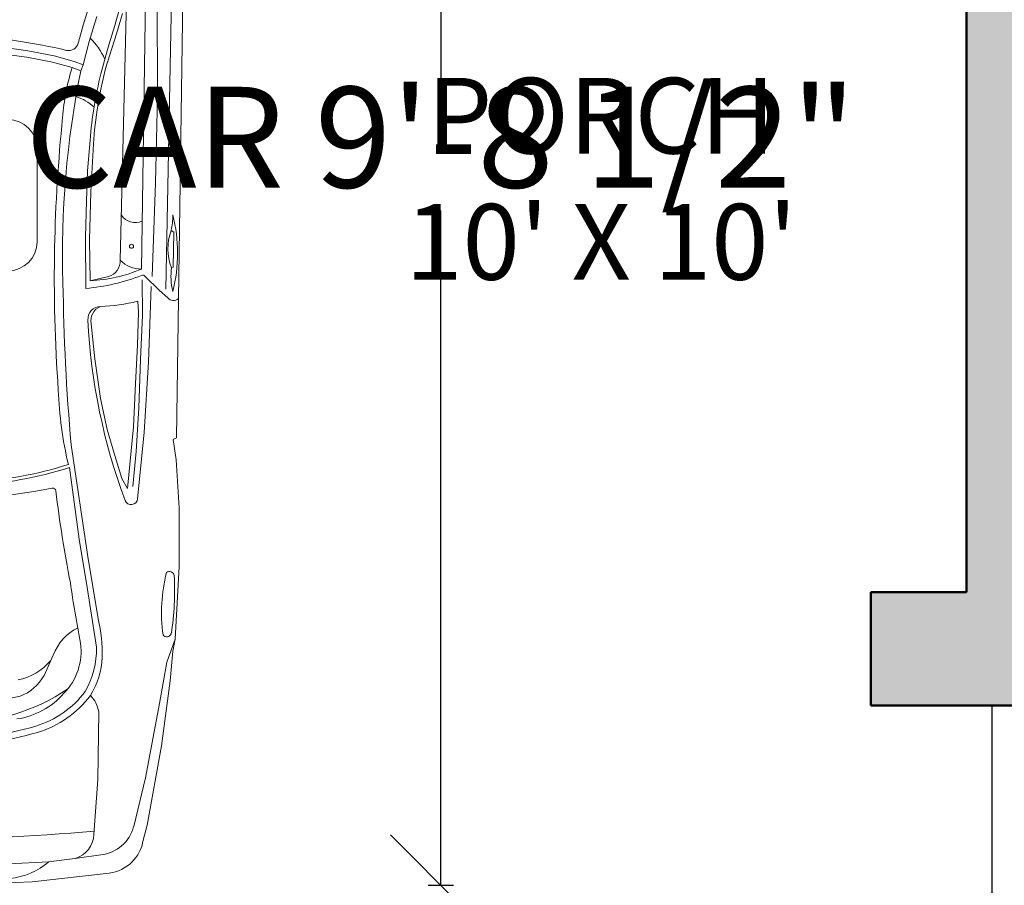
# Model space of a CAD drawing. Units: inches. Extents: x 3121 to 3511, y 1323 to 1998.
# Tile 4 of 10: x 3244 to 3322, y 1402 to 1470. Entities that reach past the tile are written whole.
import ezdxf

# ---------------------------------------------------------------- set-up
doc = ezdxf.new("R2010")
doc.units = ezdxf.units.IN
for name, color, linetype, lineweight in [('0_Equip', 250, 'Continuous', 13), ('A-ANNO-DIMS', 2, 'Continuous', 18), ('A-AREA-IDEN', 7, 'Continuous', 25), ('A-FLOR', 7, 'Continuous', 25), ('A-WALL', 7, 'Continuous', 50), ('A-WALL-PATT', 3, 'Continuous', 13)]:
    doc.layers.add(name, color=color, linetype=linetype, lineweight=lineweight)
doc.styles.get("Standard").update_dxf_attribs({"font": 'arial.ttf'})
doc.dimstyles.new('ISO-25', dxfattribs={"dimtxt": 8, "dimasz": 8, "dimexe": 1, "dimexo": 1, "dimtad": 0, "dimtih": 1, "dimtoh": 1, "dimlunit": 3, "dimtxsty": 'Standard', "dimblk": 'OBLIQUE', "dimcen": 2.5, "dimclrt": 1, "dimadec": 0, "dimazin": 0, "dimtfac": 1, "dimtmove": 0, "dimatfit": 3, "dimfxl": 1, "dimfxlon": 1, "dimarcsym": 0})

# ---------------------------------------------------------------- blocks, each defined once
blk = doc.blocks.new('A$C4C7B54D1')
at = {"layer": '0_Equip', "ltscale": 0.1}
for p, q in [((0.0322, -0.0735), (0.0457, 0.863)), ((0.0824, 0.8406), (0.0842, 0.484)), ((0.1292, 0.8299), (0.111, -0.138)), ((0.1658, 0.8152), (0.145, -0.6171)), ((-0.0162, 0.792), (-0.0361, -0.045)), ((-0.1417, 0.7577), (-0.156, 0.7129)), ((-0.1363, 0.66), (-0.1112, 0.7406)), ((-0.0287, 0.7503), (-0.0484, 0.6849)), ((-0.156, 0.7129), (-0.1712, 0.6573)), ((-0.0484, 0.6849), (-0.0834, 0.5729)), ((-0.4076, 0.6403), (-0.3337, 0.6302)), ((-0.1712, 0.6573), (-0.1719, 0.6546)), ((-0.1562, 0.5849), (-0.1363, 0.66)), ((-0.4102, 0.6196), (-0.3371, 0.6096)), ((-0.3371, 0.6096), (-0.2541, 0.593)), ((-0.3337, 0.6302), (-0.2492, 0.6133)), ((-0.2492, 0.6133), (-0.185, 0.5956)), ((-0.2541, 0.593), (-0.1914, 0.5757)), ((-0.1914, 0.5757), (-0.1635, 0.5653)), ((-0.185, 0.5956), (-0.1562, 0.5849)), ((-0.1635, 0.5653), (-0.1562, 0.5849)), ((-0.0834, 0.5729), (-0.0986, 0.5066)), ((-0.0986, 0.5066), (-0.1102, 0.4394)), ((0.0842, 0.484), (0.0779, 0.2045)), ((-0.1102, 0.4394), (-0.1192, 0.3749)), ((-0.1192, 0.3749), (-0.1228, 0.3301)), ((-0.1335, 0.3418), (-0.1413, 0.2426)), ((-0.1228, 0.3301), (-0.1309, 0.1751)), ((-0.3045, 0.3145), (-0.3045, 0.0145)), ((-0.1413, 0.2426), (-0.1454, 0.1454)), ((0.0779, 0.2045), (0.0672, -0.0974)), ((-0.1309, 0.1751), (-0.1349, 0.0193)), ((-0.1454, 0.1454), (-0.1478, 0.0305)), ((0.1285, 0.0505), (0.1365, 0.0456)), ((0.1365, 0.0456), (0.1349, -0.0676)), ((-0.1478, 0.0305), (-0.147, -0.1358)), ((-0.1349, 0.0193), (-0.1335, -0.1112)), ((0.1349, -0.0676), (0.1293, -0.0692)), ((-0.0739, -0.0972), (-0.1335, -0.1112)), ((0.0344, -0.1082), (0.0352, -0.2223)), ((0.0435, -0.0965), (0.0899, -0.143)), ((0.0633, -0.1299), (0.0545, -0.3725)), ((0.0899, -0.143), (0.1172, -0.1663)), ((0.02, -0.1773), (0.0224, -0.2127)), ((0.0224, -0.2127), (0.0192, -0.3187)), ((-0.1302, -0.2496), (-0.1182, -0.3629)), ((0.0352, -0.2223), (0.0296, -0.3653)), ((0.0192, -0.3187), (0.0135, -0.4424)), ((-0.1182, -0.3629), (-0.0997, -0.4906)), ((0.0296, -0.3653), (0.0232, -0.5203)), ((0.0545, -0.3725), (0.0408, -0.6007)), ((0.0135, -0.4424), (0.0063, -0.5822)), ((-0.0997, -0.4906), (-0.0788, -0.5902)), ((0.0232, -0.5203), (0.0151, -0.6617)), ((-0.0788, -0.5902), (-0.0571, -0.6641)), ((0.0063, -0.5822), (-0.013, -0.7806)), ((0.0408, -0.6007), (0.0198, -0.814)), ((0.145, -0.6171), (0.1349, -0.6228)), ((0.1349, -0.6228), (0.1436, -0.6885)), ((-0.1419, -0.9936), (-0.1944, -0.6398)), ((-0.0571, -0.6641), (-0.0314, -0.7485)), ((0.0151, -0.6617), (0.0039, -0.7742)), ((0.1436, -0.6885), (0.1537, -0.843)), ((-0.1898, -0.7846), (-0.2003, -0.7134)), ((-0.0314, -0.7485), (-0.013, -0.7806)), ((-0.1688, -0.9445), (-0.1898, -0.7846)), ((0.1537, -0.843), (0.1537, -1.0322)), ((-0.1419, -1.1068), (-0.1688, -0.9445)), ((-0.1069, -1.2014), (-0.1419, -0.9936)), ((0.1537, -1.0322), (0.1407, -1.2661)), ((-0.1127, -1.2925), (-0.1419, -1.1068)), ((0.1137, -1.3405), (0.1407, -1.2661)), ((0.1407, -1.2661), (0.1335, -1.3051)), ((-0.2528, -1.3182), (-0.282, -1.3835)), ((0.1335, -1.3051), (0.1248, -1.4004)), ((0.0904, -1.4736), (0.1137, -1.3405)), ((0.1248, -1.4004), (0.0973, -1.6107)), ((-0.359, -1.4501), (-0.4524, -1.4699)), ((0.0448, -1.7129), (0.0904, -1.4736)), ((-0.1057, -1.5004), (-0.1081, -1.7188)), ((0.0973, -1.6107), (0.0511, -1.8663)), ((0.0071, -1.8701), (0.0448, -1.7129)), ((-0.1081, -1.7188), (-0.1209, -1.8962)), ((0.0511, -1.8663), (0.0381, -1.914)), ((-0.1746, -1.9721), (-0.0987, -1.9616)), ((-0.3964, -1.9908), (-0.2668, -1.9838)), ((-0.2668, -1.9838), (-0.1746, -1.9721)), ((-0.0716, -2.0208), (-0.3199, -2.0483)), ((-0.3199, -2.0483), (-0.5711, -2.0598))]:
    blk.add_line(p, q, dxfattribs=at)
blk.add_circle((0, 0), 0.00662, dxfattribs=at)
for centre, radius, start, end in [((5.1546, -0.8606), 5.4408, 159.4549, 164.9096), ((-0.6617, -1.2957), 1.9795, 76.7955, 85.9193), ((-0.2978, 0.5061), 0.2334, 24.5951, 45.0123), ((-0.2023, 0.662), 0.0314, 256.7955, 346.333), ((0.5512, 0.3511), 0.7759, 163.1704, 175.2741), ((2.7585, -0.0242), 2.9809, 168.5936, 181.8095), ((1.1821, 0.2371), 1.3197, 166.0203, 175.4502), ((-0.2189, 0.3484), 0.1397, 45.3353, 73.3832), ((5.1081, -0.126), 5.3575, 174.2048, 178.6841), ((-0.3986, 0.3145), 0.0941, 0, 90), ((0.0121, 0.1296), 0.0534, 213.0531, 294.7204), ((-0.1448, 0.102), 0.2781, 349.3166, 359.8064), ((-0.3569, -0.0222), 0.5055, 345.8807, 14.1193), ((0.2762, -0.0084), 0.159, 158.2665, 202.5024), ((-0.3986, 0.0145), 0.0941, 270, 0), ((5.1217, -0.0941), 5.3705, 179.0277, 183.9499), ((-0.0879, -0.0473), 0.0519, 285.7324, 2.5463), ((0.0317, 0.0214), 0.095, 224.3815, 270.2828), ((-0.2038, 0.5164), 0.6547, 274.9778, 291.1402), ((-0.1545, 0.3651), 0.4767, 272.5286, 293.0615), ((0.0361, -0.1039), 0.0105, 44.9904, 111.1402), ((0.3303, -0.0969), 0.2029, 172.1581, 193.8654), ((6.5785, -0.0355), 6.7998, 180.69786, 185.09877), ((-0.1152, 0.3542), 0.5484, 271.5928, 284.2653), ((0.1355, -0.1514), 0.0236, 219.2612, 312.7091), ((-0.0988, -0.2358), 0.0418, 91.5928, 182.857), ((-0.0814, -0.2402), 0.0497, 111.8936, 190.9619), ((1.797, -0.1412), 1.9399, 182.857, 200.46), ((1.0027, -0.4173), 1.2396, 182.1599, 193.3442), ((-0.5926, 0.5276), 1.291, 273.3012, 287.5434), ((-0.5926, 0.5276), 1.3014, 273.2957, 287.5434), ((-0.7372, 1.7227), 2.5481, 270.2587, 280.8811), ((-0.2542, -0.7899), 0.0105, 6.8329, 100.8811), ((3.6366, -0.3237), 3.9082, 186.8329, 191.2274), ((-0.001, -0.812), 0.0209, 200.46, 354.3741), ((0.625, -1.1812), 0.5281, 165.7822, 187.813), ((0.1224, -1.0639), 0.0155, 11.61, 127.0083), ((-0.7003, -1.1122), 0.8395, 350.5693, 3.5107), ((3.2772, -0.6026), 3.5073, 187.8997, 191.1299), ((-0.6326, -1.3185), 0.5386, 359.2898, 12.5553), ((-0.0922, -1.3822), 0.1728, 118.0568, 158.2568), ((0.1138, -1.243), 0.0156, 219.7819, 334.4738), ((-0.3561, -1.3051), 0.1937, 315.5733, 7.5686), ((-0.3902, -1.2979), 0.2775, 330.2938, 1.1189), ((-0.3569, -1.3104), 0.2633, 328.496, 356.7864), ((-0.4032, -1.2146), 0.1871, 281.6041, 319.5969), ((-0.4092, -1.3141), 0.145, 290.2682, 331.3813), ((-0.5601, -0.9022), 0.6331, 268.9773, 304.1276), ((-0.4054, -1.2776), 0.2487, 278.3054, 318.9935), ((-0.3993, -1.2472), 0.313, 286.7946, 323.0516), ((-0.3993, -1.2472), 0.3339, 286.7686, 323.0516), ((-0.2012, -1.516), 0.0967, 9.2726, 44.7049), ((-0.6629, -0.3101), 1.2865, 272.754, 285.9737), ((-0.6629, -0.3101), 1.3074, 272.7319, 285.9802), ((-0.1121, -1.8393), 0.123, 276.2164, 345.5014), ((-0.938, 7.9307), 9.8503, 271.23497, 274.76255), ((-0.2061, -1.8915), 0.0853, 287.3595, 356.7945), ((-0.0885, -1.8937), 0.1282, 277.5847, 350.907), ((-0.41, -1.8225), 0.2157, 274.5609, 311.594)]:
    blk.add_arc(centre, radius, start, end, dxfattribs=at)
blk = doc.blocks.new('_Oblique')
at = {"color": 0, "linetype": 'ByBlock', "lineweight": -2}
blk.add_line((-0.5, -0.5), (0.5, 0.5), dxfattribs=at)
blk = doc.blocks.new('*D31')
at = {"layer": 'A-ANNO-DIMS', "color": 0, "lineweight": -2, "transparency": 16777216}
for p, q in [((3276.231, 1518.068), (3278.231, 1518.068)), ((3277.231, 1518.068), (3277.231, 1464.563)), ((3277.231, 1401.535), (3277.231, 1455.04)), ((3276.231, 1401.535), (3278.231, 1401.535))]:
    blk.add_line(p, q, dxfattribs=at)
at = {"layer": 'Defpoints', "color": 0, "transparency": 16777216}
for p in [(3259.751, 1518.068), (3277.231, 1518.068), (3259.751, 1401.535)]:
    blk.add_point(p, dxfattribs=at)
at = {"layer": 'A-ANNO-DIMS', "color": 0, "lineweight": -2, "transparency": 16777216, "xscale": 8, "yscale": 8, "zscale": 8}
for p, rotation in [((3277.231, 1518.068), 90), ((3277.231, 1401.535), 270)]:
    blk.add_blockref('_Oblique', p, dxfattribs=dict(at, rotation=rotation))
at = {"layer": 'A-ANNO-DIMS', "color": 1, "transparency": 16777216, "insert": (3277.231, 1459.801), "char_height": 8, "attachment_point": 5}
blk.add_mtext('CAR 9\'-8 1/2"', dxfattribs=at)
blk = doc.blocks.new('*D53')
at = {"layer": 'A-ANNO-DIMS', "color": 0, "lineweight": -2, "transparency": 16777216}
for p, q in [((3274.023, 1336.367), (3274.023, 1334.367)), ((3310.023, 1336.367), (3310.023, 1334.367)), ((3274.023, 1335.367), (3280.768, 1335.367)), ((3310.023, 1335.367), (3303.278, 1335.367))]:
    blk.add_line(p, q, dxfattribs=at)
at = {"layer": 'Defpoints', "color": 0, "transparency": 16777216}
for p in [(3274.023, 1946.784), (3310.023, 1946.784), (3310.023, 1335.367)]:
    blk.add_point(p, dxfattribs=at)
at = {"layer": 'A-ANNO-DIMS', "color": 0, "lineweight": -2, "transparency": 16777216, "xscale": 8, "yscale": 8, "zscale": 8, "rotation": 180}
blk.add_blockref('_Oblique', (3274.023, 1335.367), dxfattribs=at)
at = {"layer": 'A-ANNO-DIMS', "color": 0, "lineweight": -2, "transparency": 16777216, "xscale": 8, "yscale": 8, "zscale": 8}
blk.add_blockref('_Oblique', (3310.023, 1335.367), dxfattribs=at)
at = {"layer": 'A-ANNO-DIMS', "color": 1, "transparency": 16777216, "insert": (3292.023, 1335.367), "char_height": 8, "attachment_point": 5}
blk.add_mtext('3\'-0"', dxfattribs=at)
blk = doc.blocks.new('*D54')
at = {"layer": 'A-ANNO-DIMS', "color": 0, "lineweight": -2, "transparency": 16777216}
for p, q in [((3310.023, 1336.367), (3310.023, 1334.367)), ((3334.156, 1336.367), (3334.156, 1334.367)), ((3310.023, 1335.367), (3310.763, 1335.367)), ((3334.156, 1335.367), (3333.416, 1335.367))]:
    blk.add_line(p, q, dxfattribs=at)
at = {"layer": 'Defpoints', "color": 0, "transparency": 16777216}
for p in [(3310.023, 1946.784), (3334.156, 1946.784), (3334.156, 1335.367)]:
    blk.add_point(p, dxfattribs=at)
at = {"layer": 'A-ANNO-DIMS', "color": 0, "lineweight": -2, "transparency": 16777216, "xscale": 8, "yscale": 8, "zscale": 8, "rotation": 180}
blk.add_blockref('_Oblique', (3310.023, 1335.367), dxfattribs=at)
at = {"layer": 'A-ANNO-DIMS', "color": 0, "lineweight": -2, "transparency": 16777216, "xscale": 8, "yscale": 8, "zscale": 8}
blk.add_blockref('_Oblique', (3334.156, 1335.367), dxfattribs=at)
at = {"layer": 'A-ANNO-DIMS', "color": 1, "transparency": 16777216, "insert": (3322.089, 1335.367), "char_height": 8, "attachment_point": 5}
blk.add_mtext('2\'-0"', dxfattribs=at)
blk = doc.blocks.new('*D58')
at = {"layer": 'A-ANNO-DIMS', "color": 0, "lineweight": -2, "transparency": 16777216}
for p, q in [((3209.892, 1985.334), (3209.892, 1987.334)), ((3311.328, 1985.334), (3311.328, 1987.334)), ((3209.892, 1986.334), (3240.026, 1986.334)), ((3311.328, 1986.334), (3281.194, 1986.334))]:
    blk.add_line(p, q, dxfattribs=at)
at = {"layer": 'Defpoints', "color": 0, "transparency": 16777216}
for p in [(3311.328, 1986.334), (3209.892, 1424.784), (3311.328, 1424.784)]:
    blk.add_point(p, dxfattribs=at)
at = {"layer": 'A-ANNO-DIMS', "color": 0, "lineweight": -2, "transparency": 16777216, "xscale": 8, "yscale": 8, "zscale": 8, "rotation": 180}
blk.add_blockref('_Oblique', (3209.892, 1986.334), dxfattribs=at)
at = {"layer": 'A-ANNO-DIMS', "color": 0, "lineweight": -2, "transparency": 16777216, "xscale": 8, "yscale": 8, "zscale": 8}
blk.add_blockref('_Oblique', (3311.328, 1986.334), dxfattribs=at)
at = {"layer": 'A-ANNO-DIMS', "color": 1, "transparency": 16777216, "insert": (3260.61, 1986.334), "char_height": 8, "attachment_point": 5}
blk.add_mtext('8\'-5 1/2"', dxfattribs=at)
blk = doc.blocks.new('*D59')
at = {"layer": 'A-ANNO-DIMS', "color": 0, "lineweight": -2, "transparency": 16777216}
for p, q in [((3318.918, 1336.367), (3318.918, 1334.367)), ((3370.918, 1336.367), (3370.918, 1334.367)), ((3318.918, 1335.367), (3333.499, 1335.367)), ((3370.918, 1335.367), (3356.337, 1335.367))]:
    blk.add_line(p, q, dxfattribs=at)
at = {"layer": 'Defpoints', "color": 0, "transparency": 16777216}
for p in [(3318.918, 1752.226), (3370.918, 1748.784), (3370.918, 1335.367)]:
    blk.add_point(p, dxfattribs=at)
at = {"layer": 'A-ANNO-DIMS', "color": 0, "lineweight": -2, "transparency": 16777216, "xscale": 8, "yscale": 8, "zscale": 8, "rotation": 180}
blk.add_blockref('_Oblique', (3318.918, 1335.367), dxfattribs=at)
at = {"layer": 'A-ANNO-DIMS', "color": 0, "lineweight": -2, "transparency": 16777216, "xscale": 8, "yscale": 8, "zscale": 8}
blk.add_blockref('_Oblique', (3370.918, 1335.367), dxfattribs=at)
at = {"layer": 'A-ANNO-DIMS', "color": 1, "transparency": 16777216, "insert": (3344.918, 1335.367), "char_height": 8, "attachment_point": 5}
blk.add_mtext('4\'-4"', dxfattribs=at)
blk = doc.blocks.new('*D73')
at = {"layer": 'A-ANNO-DIMS', "color": 0, "lineweight": -2, "transparency": 16777216}
for p, q in [((3261.023, 1336.367), (3261.023, 1334.367)), ((3301.026, 1336.367), (3301.026, 1334.367)), ((3261.023, 1335.367), (3269.769, 1335.367)), ((3301.026, 1335.367), (3292.28, 1335.367))]:
    blk.add_line(p, q, dxfattribs=at)
at = {"layer": 'Defpoints', "color": 0, "transparency": 16777216}
for p in [(3261.023, 1739.784), (3301.026, 1739.784), (3301.026, 1335.367)]:
    blk.add_point(p, dxfattribs=at)
at = {"layer": 'A-ANNO-DIMS', "color": 0, "lineweight": -2, "transparency": 16777216, "xscale": 8, "yscale": 8, "zscale": 8, "rotation": 180}
blk.add_blockref('_Oblique', (3261.023, 1335.367), dxfattribs=at)
at = {"layer": 'A-ANNO-DIMS', "color": 0, "lineweight": -2, "transparency": 16777216, "xscale": 8, "yscale": 8, "zscale": 8}
blk.add_blockref('_Oblique', (3301.026, 1335.367), dxfattribs=at)
at = {"layer": 'A-ANNO-DIMS', "color": 1, "transparency": 16777216, "insert": (3281.024, 1335.367), "char_height": 8, "attachment_point": 5}
blk.add_mtext('3\'-4"', dxfattribs=at)

msp = doc.modelspace()

# ---------------------------------------------------------------- hatches: boundary and pattern name
at = {"layer": 'A-WALL-PATT'}
h = msp.add_hatch(color=256, dxfattribs=at)
h.dxf.hatch_style = 1
h.paths.add_polyline_path([(3274.023, 1955.784), (3189.918, 1955.784), (3189.918, 1910.219), (3198.918, 1910.219), (3198.918, 1946.784), (3259.023, 1946.784), (3259.023, 1921.61), (3261.023, 1921.61), (3261.023, 1946.784), (3274.023, 1946.784)])
h.paths.add_polyline_path([(3327.918, 1946.784), (3334.156, 1946.784), (3334.156, 1955.784), (3310.023, 1955.784), (3310.023, 1946.784), (3318.918, 1946.784), (3318.918, 1929.796), (3311.644, 1929.796), (3311.644, 1927.007), (3324.033, 1927.007), (3324.033, 1871.381), (3311.644, 1871.381), (3311.644, 1868.381), (3318.918, 1868.381), (3318.918, 1853.784), (3327.918, 1853.784)])
h.paths.add_polyline_path([(3456.918, 1955.784), (3384.562, 1955.784), (3384.562, 1946.784), (3447.918, 1946.784), (3447.918, 1877.779), (3456.918, 1877.779)])
h.paths.add_polyline_path([(3456.918, 1835.782), (3447.918, 1835.782), (3447.918, 1814.784), (3414.918, 1814.784), (3414.918, 1803.784), (3447.918, 1803.784), (3447.918, 1793.443), (3456.918, 1793.443)])
h.paths.add_polyline_path([(3456.918, 1558.434), (3447.918, 1558.434), (3447.918, 1547.784), (3375.918, 1547.784), (3375.918, 1598.784), (3378.918, 1598.784), (3378.918, 1602.284), (3375.918, 1602.284), (3375.918, 1674.284), (3369.918, 1674.284), (3369.918, 1547.784), (3364.418, 1547.784), (3364.418, 1538.784), (3447.918, 1538.784), (3447.918, 1512.628), (3456.918, 1512.628)])
h.paths.add_polyline_path([(3456.918, 1460.558), (3447.918, 1460.558), (3447.918, 1424.784), (3412.543, 1424.784), (3412.543, 1415.784), (3456.918, 1415.784)])
h.paths.add_polyline_path([(3358.149, 1424.784), (3322.918, 1424.784), (3322.918, 1538.784), (3328.418, 1538.784), (3328.418, 1547.784), (3308.208, 1547.784), (3308.208, 1538.784), (3318.918, 1538.784), (3318.918, 1424.784), (3311.328, 1424.784), (3311.328, 1415.784), (3358.149, 1415.784)])
h.paths.add_polyline_path([(3207.562, 1547.784), (3198.918, 1547.784), (3198.918, 1607.327), (3189.918, 1607.327), (3189.918, 1513.073), (3198.918, 1513.073), (3198.918, 1538.784), (3207.562, 1538.784)])
h.paths.add_polyline_path([(3198.918, 1461.548), (3189.918, 1461.548), (3189.918, 1415.784), (3209.892, 1415.784), (3209.892, 1424.784), (3198.918, 1424.784)])
h.paths.add_polyline_path([(3272.208, 1547.784), (3238.766, 1547.784), (3238.766, 1538.784), (3272.208, 1538.784)])
h.paths.add_polyline_path([(3261.023, 1748.784), (3198.918, 1748.784), (3198.918, 1768.387), (3189.918, 1768.387), (3189.918, 1692.279), (3198.918, 1692.279), (3198.918, 1739.784), (3261.023, 1739.784)])
h.paths.add_polyline_path([(3198.918, 1856.171), (3189.918, 1856.171), (3189.918, 1808.331), (3198.918, 1808.331), (3198.918, 1821.074), (3261.023, 1821.074), (3261.023, 1862.309), (3259.023, 1862.309), (3259.023, 1825.074), (3198.918, 1825.074)])

# ---------------------------------------------------------------- linework, layer by layer
at = {"layer": 'A-FLOR'}
msp.add_lwpolyline([(3320.918, 1415.784), (3320.918, 1367.917), (3191.918, 1367.917), (3191.918, 1415.784)], dxfattribs=at)
at = {"layer": 'A-WALL'}
for p, q in [((3318.918, 1424.784), (3318.918, 1538.784)), ((3311.328, 1424.784), (3311.328, 1415.784)), ((3311.328, 1424.784), (3318.918, 1424.784)), ((3311.328, 1415.784), (3456.918, 1415.784))]:
    msp.add_line(p, q, dxfattribs=at)

# ---------------------------------------------------------------- block references
at = {"layer": '0_Equip', "xscale": 24.59625072819005, "yscale": 24.59625072819005, "zscale": 24.59625072819005}
msp.add_blockref('A$C4C7B54D1', (3252.699, 1452.199), dxfattribs=at)

# ---------------------------------------------------------------- texts
at = {"layer": 'A-AREA-IDEN', "insert": (3268.171, 1465.549), "char_height": 6, "attachment_point": 1}
msp.add_mtext_dynamic_manual_height_columns("\\pxqc;PORCH\\P10' X 10'", width=43.56631, gutter_width=12.5, heights=[0], dxfattribs=at)

# ---------------------------------------------------------------- dimensions: what is measured, and where the dimension line sits
at = {"layer": 'A-ANNO-DIMS'}
for base, p1, p2, picture, middle in [((3311.328, 1986.334), (3209.892, 1424.784), (3311.328, 1424.784), '*D58', (3260.61, 1986.334)), ((3310.023, 1335.367), (3274.023, 1946.784), (3310.023, 1946.784), '*D53', (3292.023, 1335.367)), ((3334.156, 1335.367), (3310.023, 1946.784), (3334.156, 1946.784), '*D54', (3322.089, 1335.367)), ((3370.918, 1335.367), (3318.918, 1752.226), (3370.918, 1748.784), '*D59', (3344.918, 1335.367)), ((3301.026, 1335.367), (3261.023, 1739.784), (3301.026, 1739.784), '*D73', (3281.024, 1335.367))]:
    dim = msp.add_linear_dim(base=base, p1=p1, p2=p2, dimstyle='ISO-25', override={"dimdec": 1, "dimlfac": 1, "dimrnd": 0, "dimzin": 1, "dimdsep": 46, "dimlunit": 4, "dimfrac": 2}, dxfattribs=at)
    dim.commit()
    dim.dimension.update_dxf_attribs({"geometry": picture, "text_midpoint": middle})
dim = msp.add_linear_dim(base=(3277.231, 1518.068), p1=(3259.751, 1401.535), p2=(3259.751, 1518.068), angle=90, text='CAR <>', dimstyle='ISO-25', override={"dimdec": 1, "dimlfac": 1, "dimrnd": 0, "dimzin": 1, "dimdsep": 46, "dimlunit": 4, "dimfrac": 2}, dxfattribs=at)
dim.commit()
dim.dimension.update_dxf_attribs({"geometry": '*D31', "text_midpoint": (3277.231, 1459.801)})

doc.saveas('drawing.dxf')
